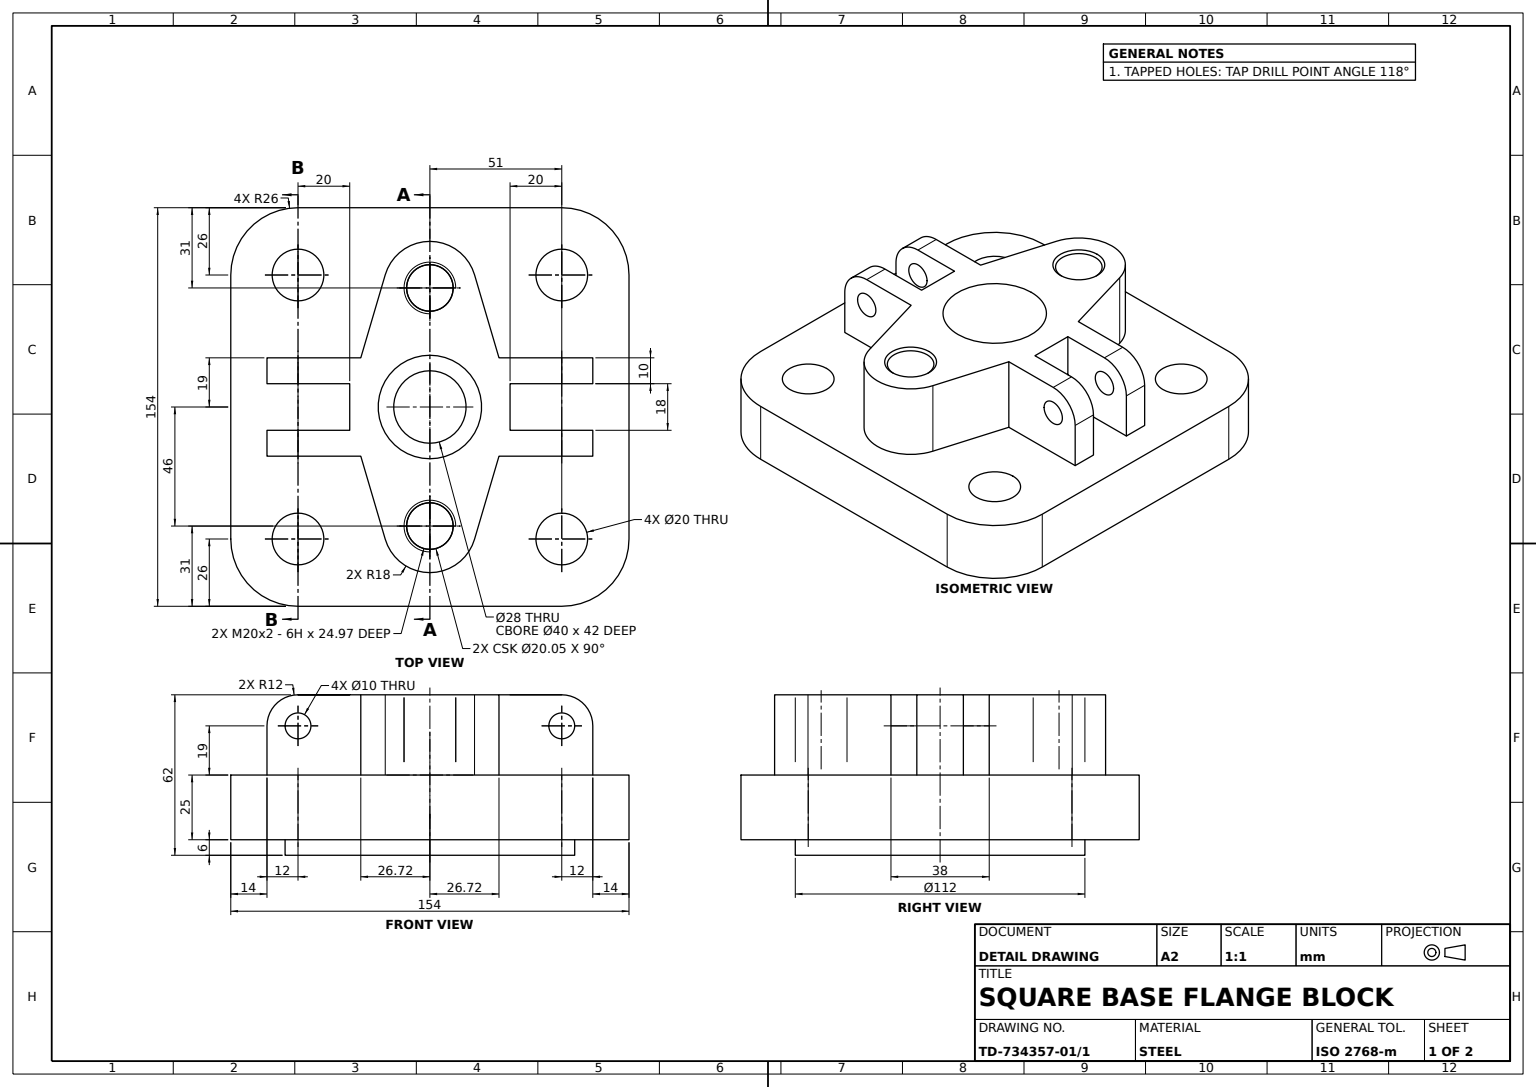
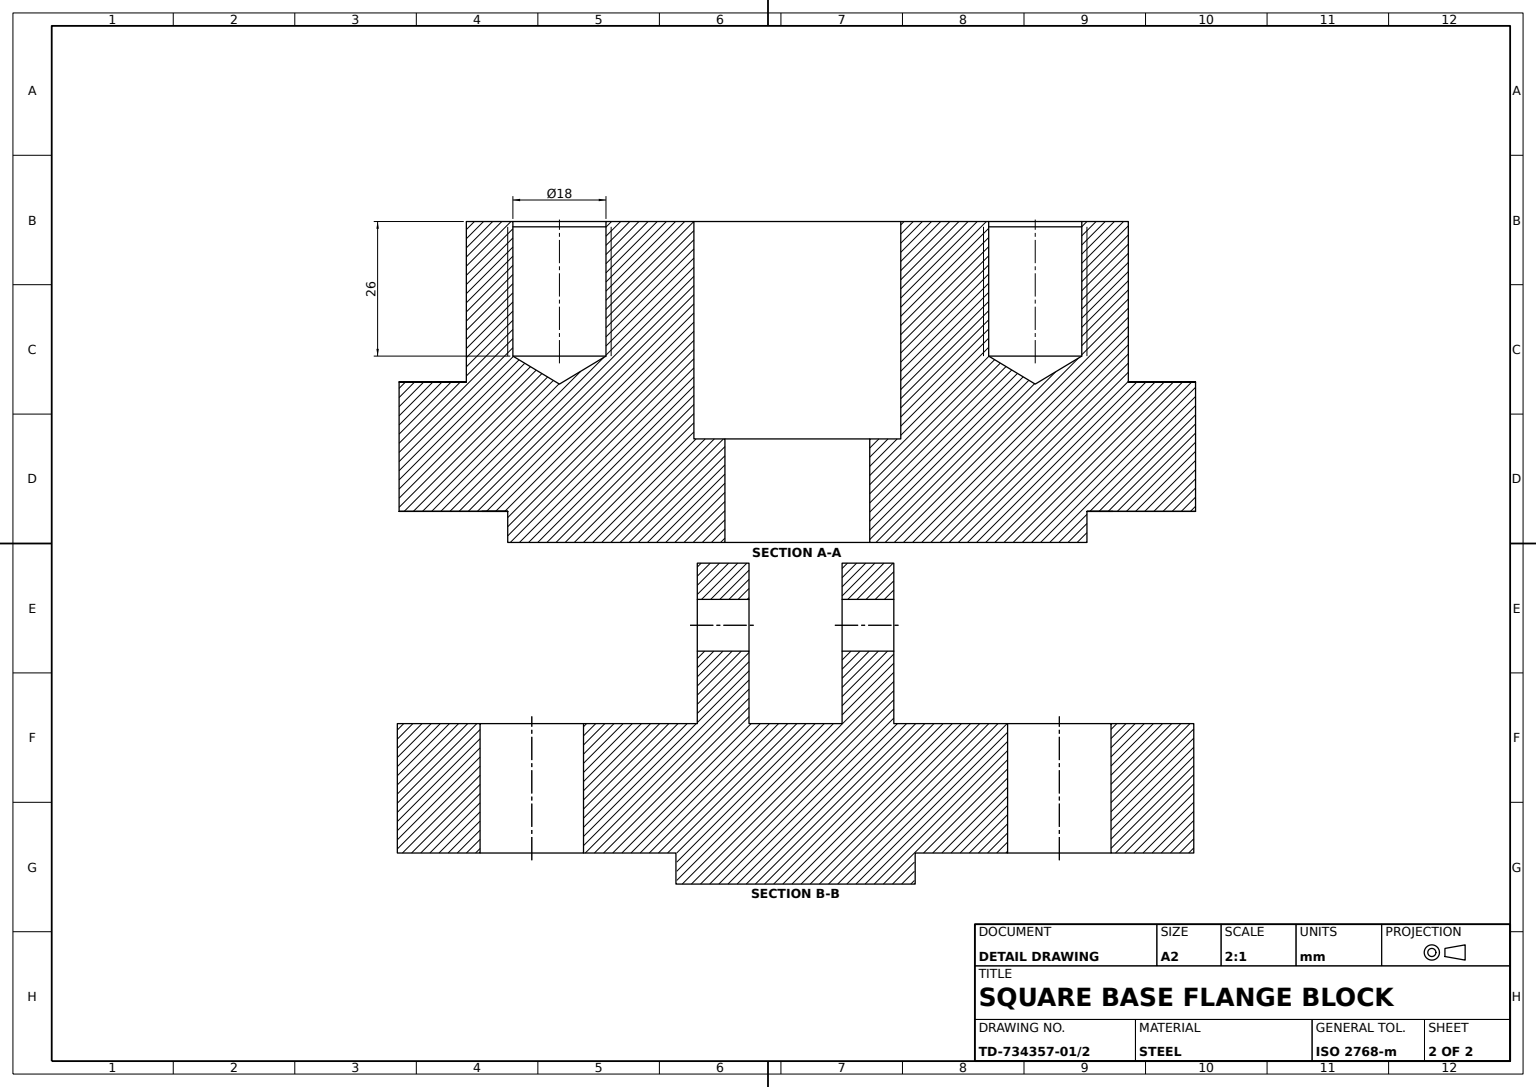
SolidWorks part; units mm, degrees
material "Plain Carbon Steel"
ref_plane "Front Plane" through (0, 0, 0) normal (0, 0, 1) x (1, 0, 0)
ref_plane "Top Plane" through (0, 0, 0) normal (0, 1, 0) x (1, 0, 0)
ref_plane "Right Plane" through (0, 0, 0) normal (1, 0, 0) x (0, 0, -1)
sketch "Base Plate Profile 154x154 R26" plane through (0, 0, 0) normal (0, 1, 0) x (1, 0, 0)
  line L1 (-51, -77) -> (51, -77)
  line L2 (-77, -51) -> (-77, 51)
  line L3 (-51, 77) -> (51, 77)
  line L4 (77, -51) -> (77, 51)
  line L5 (-77, -77) -> (77, 77) construction
  line L6 (-77, 77) -> (77, -77) construction
  arc A0 (-51, -77) -> (-77, -51) centre (-51, -51) cw
  arc A1 (51, -77) -> (77, -51) centre (51, -51) ccw
  arc A2 (51, 77) -> (77, 51) centre (51, 51) cw
  arc A3 (-77, 51) -> (-51, 77) centre (-51, 51) cw
  point P0 (0, 0)
  dimension "D3" = 26
  dimension "D1" = 154
  dimension "D2" = 154
extrude "Base Plate 154x154x25" add sketch "Base Plate Profile 154x154 R26" along normal blind 25
sketch "Locating Spigot Sketch Ø112" plane through (0, 0, 0) normal (0, -1, 0) x (1, 0, 0)
  circle A0 centre (0, 0) radius 56
  dimension "D1" = 112
extrude "Locating Spigot Ø112x6" add sketch "Locating Spigot Sketch Ø112" along normal blind 6
sketch "Pivot Boss Profile" plane through (0, 25, 0) normal (0, 1, 0) x (1, 0, 0)
  line L0 (-77, 51) -> (-77, -51) construction
  line L1 (77, -51) -> (77, 51) construction
  line L2 (-17.2662, 51.087) -> (-26.7197, 19)
  line L3 (17.2662, 51.087) -> (26.7197, 19)
  line L4 (-17.2662, -51.087) -> (-26.7197, -19)
  line L5 (17.2662, -51.087) -> (26.7197, -19)
  line L6 (-31, -9) -> (-31, 9)
  line L7 (-31, 9) -> (-63, 9)
  line L8 (-63, 9) -> (-63, 19)
  line L9 (-63, 19) -> (-26.7197, 19)
  line L10 (0, 0) -> (-31, 0) construction
  line L11 (-63, -19) -> (-26.7197, -19)
  line L12 (-63, -9) -> (-63, -19)
  line L13 (-31, -9) -> (-63, -9)
  line L15 (63, -19) -> (26.7197, -19)
  line L16 (63, -9) -> (63, -19)
  line L17 (31, -9) -> (63, -9)
  line L18 (31, -9) -> (31, 9)
  line L19 (63, 9) -> (63, 19)
  line L20 (31, 9) -> (63, 9)
  line L21 (63, 19) -> (26.7197, 19)
  arc A1 (17.2662, 51.087) -> (-17.2662, 51.087) centre (0, 46) ccw
  arc A2 (-17.2662, -51.087) -> (17.2662, -51.087) centre (0, -46) ccw
  dimension "D2" = 36
  dimension "D3" = 46
  dimension "D4" = 46
  dimension "D5" = 77
  dimension "D6" = 77
  dimension "D7" = 9
  dimension "D8" = 14
  dimension "D9" = 63
  dimension "D10" = 19
  dimension "D11" = 63
  dimension "D12" = 19
  dimension "D13" = 18
  dimension "D14" = 26.7197
  dimension "D15" = 19
  dimension "D16" = 63
  dimension "D17" = 10
  dimension "D18" = 10
  dimension "D19" = 9
  dimension "D20" = 102.1739
  dimension "D21" = 31
  dimension "D22" = 36.2803
  dimension "D23" = 51.087
  dimension "D24" = 62
  dimension "D25" = 63
  dimension "D26" = 26.7197
  dimension "D27" = 9
extrude "Pivot Boss with Lugs" add sketch "Pivot Boss Profile" along normal blind 31
fillet "Pivot Boss Fillets R12" radius 12 4 edges at (63, 56, 14) (63, 56, -14) (-63, 56, -14) (-63, 56, 14)
sketch "Lug Pin Holes Sketch Ø10" plane through (0, 0, 19) normal (0, 0, 1) x (1, 0, 0)
  circle A0 centre (-51, 44) radius 5
  circle A1 centre (51, 44) radius 5
  dimension "D1" = 10
extrude "Lug Pin Holes Ø10" cut sketch "Lug Pin Holes Sketch Ø10" against normal through all
sketch "Centre Bore Sketch Ø40" plane through (0, 56, 0) normal (0, 1, 0) x (1, 0, 0)
  circle A0 centre (0, 0) radius 20
  dimension "D1" = 40
extrude "Centre Bore Ø40" cut sketch "Centre Bore Sketch Ø40" against normal blind 42
sketch "Through Bore Sketch Ø28" plane through (0, 14, 0) normal (0, 1, 0) x (1, 0, 0)
  circle A0 centre (0, 0) radius 14
  dimension "D1" = 28
extrude "Through Bore Ø28" cut sketch "Through Bore Sketch Ø28" against normal blind 42
hole_wizard "Tapped Holes M20x2.0" positions "Sketch7" profile "Sketch8" tap size "M20x2.0" standard "ISO"
sketch "Sketch7" plane through (0, 56, 0) normal (0, 1, 0) x (1, 0, 0)
  point P0 (0, 46)
  point P3 (0, -46)
sketch "Sketch8" plane through (0, 56, -46) normal (1, 0, 0) x (0, 0, 1)
  line L0 (0, 0) -> (0, 31.4077)
  line L1 (0, 31.4077) -> (9, 26)
  line L2 (9, 26) -> (9, 1.025)
  line L3 (9, 1.025) -> (10.025, 0)
  line L5 (10.025, 0) -> (0, 0)
  line L6 (-9, 1.025) -> (-10.025, 0) construction
  line L10 (0, 31.4077) -> (-9, 26) construction
  line L11 (0, -6.35) -> (0, 107.95) construction
  dimension "Tap Drill Dia." = 18
  dimension "Tap Drill Depth" = 26
  dimension "Near C'Sink Dia." = 20.05
  dimension "Near C'Sink Angle" = 90
  dimension "Drill Angle" = 118
cosmetic thread "Hole Thread1" parameters "D1"=40, "D2"=20
cosmetic thread "Hole Thread2" parameters "D1"=40, "D2"=20
sketch "Mounting Holes Sketch 4xØ20" plane through (0, 25, 0) normal (0, 1, 0) x (1, 0, 0)
  circle A0 centre (51, 51) radius 10
  circle A1 centre (-51, 51) radius 10
  circle A2 centre (-51, -51) radius 10
  circle A3 centre (51, -51) radius 10
  dimension "D1" = 20
extrude "Mounting Holes 4xØ20" cut sketch "Mounting Holes Sketch 4xØ20" against normal blind 42
